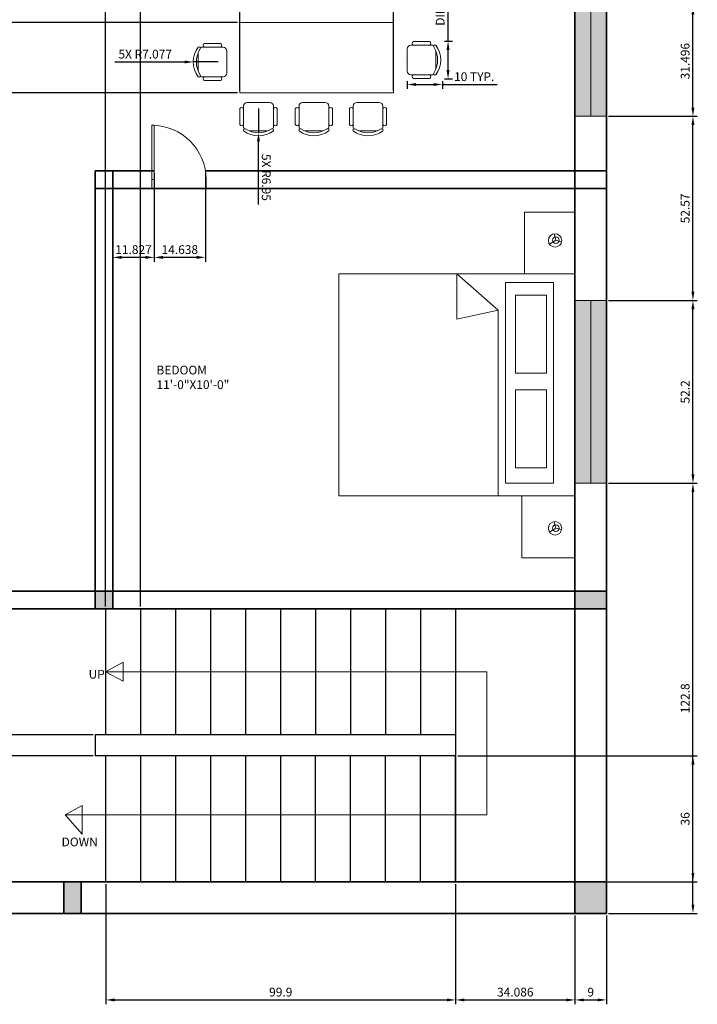
# Model space of a CAD drawing. Units: inches. Extents: x 33934 to 34340, y 20959 to 21493.
# Tile 2 of 4: x 34146 to 34340, y 20959 to 21240. Entities that reach past the tile are written whole.
import ezdxf

# ---------------------------------------------------------------- set-up
doc = ezdxf.new("R2010")
doc.units = ezdxf.units.IN
for name, color, linetype, lineweight in [('A-ANNO-DIMS', 2, 'Continuous', 18), ('A-ANNO-SYMB', 7, 'Continuous', 18), ('A-ANNO-TEXT', 7, 'Continuous', 18), ('A-AREA-IDEN', 7, 'Continuous', 18), ('A-COLS', 7, 'Continuous', 35), ('A-DOOR', 3, 'Continuous', 18), ('A-FLOR-STRS', 7, 'Continuous', 25), ('A-FURN', 8, 'Continuous', 18), ('A-GLAZ', 4, 'Continuous', 18), ('A-WALL', 7, 'Continuous', 35)]:
    doc.layers.add(name, color=color, linetype=linetype, lineweight=lineweight)
doc.layers.add('A-COLS-PATT', color=141, linetype='Continuous', lineweight=13, true_color=0xadddf7)
doc.layers.add('A-GLAZ-PATT', color=159, linetype='Continuous', lineweight=13, true_color=0x22346e)
doc.styles.get("Standard").update_dxf_attribs({"font": 'arial.ttf'})
doc.dimstyles.new('ISO-25', dxfattribs={"dimtxt": 2.5, "dimasz": 2.5, "dimexe": 1.25, "dimexo": 0.625, "dimtad": 1, "dimtxsty": 'Standard', "dimcen": 2.5, "dimadec": 0, "dimazin": 0, "dimtfac": 1, "dimtmove": 0, "dimatfit": 3, "dimfxl": 1, "dimarcsym": 0})

# ---------------------------------------------------------------- blocks, each defined once
blk = doc.blocks.new('CHAIR7')
for p, q in [((0, 9), (0, -9)), ((20, 12), (3, 12)), ((5.12, 15.04), (17.88, 15.04)), ((23, -7.44), (23, 7.44)), ((3, -12), (20, -12)), ((5.12, -15), (17.88, -15))]:
    blk.add_line(p, q)
for centre, radius, start, end in [((3, 9), 3, 90, 180), ((5.56, 13.54), 1.56, 73.7398, 286.2602), ((17.44, 13.54), 1.56, 253.7398, 106.2602), ((20, 9), 3, 62.41556, 90), ((22.34, 11.12), 1.1, 53.30994, 212.02741), ((4.82, 0), 19.64, 327.57575, 32.42425), ((7, 0), 20, 323.1301, 36.8699), ((3, -9), 3, 180, 270), ((5.56, -13.5), 1.56, 73.7398, 286.2602), ((17.44, -13.5), 1.56, 253.7398, 106.2602), ((20, -9), 3, 270, 297.58444), ((22.34, -11.12), 1.1, 147.97259, 306.69006)]:
    blk.add_arc(centre, radius, start, end)
blk = doc.blocks.new('*U5')
for p, q in [((0, 0), (0, -6)), ((40, 0), (40, -6))]:
    blk.add_line(p, q)
blk.add_lwpolyline([(0, 0), (0, 40), (1.75, 40), (1.75, 0)], close=True)
blk.add_arc((0, 0), 40, 0, 90)
blk = doc.blocks.new('BED-DOUBLE-WITH-NIGHTSTANDS')
for p, q in [((-9.63, -5.48), (-11.46, -5.95)), ((-9.63, -5.48), (-9.19, -3.82)), ((-9.63, -5.48), (-8.53, -7.28)), ((72.57, -5.48), (70.73, -5.95)), ((72.57, -5.48), (73, -3.82)), ((72.57, -5.48), (73.67, -7.28)), ((10.3, -21.96), (0, -33.74)), ((63.37, -21.96), (10.3, -21.96)), ((12.88, -33.74), (10.3, -21.96)), ((0, -33.74), (12.88, -33.74))]:
    blk.add_line(p, q)
for points in [[(-17.69, 0.01), (-0.01, 0.01), (-0.01, -14.39), (-17.69, -14.39)], [(0, 0), (63.37, 0), (63.37, -67.48), (0, -67.48)], [(63.36, 0.01), (81.04, 0.01), (81.04, -15.15), (63.36, -15.15)], [(2.46, -6.09), (59.71, -6.09), (59.71, -19.82), (2.46, -19.82)], [(6.09, -8.09), (28.36, -8.09), (28.36, -16.99), (6.09, -16.99)], [(33.05, -8.09), (55.31, -8.09), (55.31, -16.99), (33.05, -16.99)]]:
    blk.add_lwpolyline(points, close=True)
for centre, radius in [((-9.57, -5.69), 1.91), ((-9.63, -5.48), 0.951), ((72.62, -5.69), 1.91), ((72.57, -5.48), 0.951)]:
    blk.add_circle(centre, radius)
blk = doc.blocks.new('*D11')
at = {"layer": 'A-ANNO-DIMS', "color": 0, "lineweight": -2, "transparency": 16777216}
for p, q in [((34268.45, 21234.15), (34268.45, 21274.98)), ((34267.46, 21234.15), (34269.7, 21234.15)), ((34268.45, 21225.89), (34268.45, 21231.65)), ((34267.46, 21223.39), (34269.7, 21223.39))]:
    blk.add_line(p, q, dxfattribs=at)
at = {"layer": 'A-ANNO-DIMS', "color": 0, "transparency": 16777216}
for points in [[(34268.03, 21231.65), (34268.87, 21231.65), (34268.45, 21234.15)], [(34268.03, 21225.89), (34268.87, 21225.89), (34268.45, 21223.39)]]:
    blk.add_solid(points, dxfattribs=at)
at = {"layer": 'Defpoints', "color": 0, "transparency": 16777216}
for p in [(34266.83, 21234.15), (34268.45, 21234.15), (34266.83, 21223.39)]:
    blk.add_point(p, dxfattribs=at)
at = {"layer": 'A-ANNO-DIMS', "color": 0, "transparency": 16777216, "insert": (34266.53, 21255.82), "char_height": 2.5, "attachment_point": 5, "rotation": 90}
blk.add_mtext('DINING CHAIR 11 TYP.', dxfattribs=at)
blk = doc.blocks.new('*D12')
at = {"layer": 'A-ANNO-DIMS', "color": 0, "lineweight": -2, "transparency": 16777216}
for p, q in [((34256.81, 21222.77), (34256.81, 21220.53)), ((34266.83, 21222.77), (34266.83, 21220.53)), ((34259.31, 21221.78), (34264.33, 21221.78)), ((34266.83, 21221.78), (34282.52, 21221.78))]:
    blk.add_line(p, q, dxfattribs=at)
at = {"layer": 'A-ANNO-DIMS', "color": 0, "transparency": 16777216}
for points in [[(34259.31, 21222.19), (34259.31, 21221.36), (34256.81, 21221.78)], [(34264.33, 21222.19), (34264.33, 21221.36), (34266.83, 21221.78)]]:
    blk.add_solid(points, dxfattribs=at)
at = {"layer": 'Defpoints', "color": 0, "transparency": 16777216}
for p in [(34256.81, 21223.39), (34266.83, 21223.39), (34266.83, 21221.78)]:
    blk.add_point(p, dxfattribs=at)
at = {"layer": 'A-ANNO-DIMS', "color": 0, "transparency": 16777216, "insert": (34275.93, 21223.68), "char_height": 2.5, "attachment_point": 5}
blk.add_mtext('10 TYP.', dxfattribs=at)
blk = doc.blocks.new('*D23')
at = {"layer": 'A-ANNO-DIMS', "color": 0, "lineweight": -2, "transparency": 16777216}
for p, q in [((34314.32, 21107.92), (34339.64, 21107.92)), ((34338.39, 20987.61), (34338.39, 21105.42)), ((34314.32, 20985.11), (34339.64, 20985.11))]:
    blk.add_line(p, q, dxfattribs=at)
at = {"layer": 'A-ANNO-DIMS', "color": 0, "transparency": 16777216}
for points in [[(34337.98, 21105.42), (34338.81, 21105.42), (34338.39, 21107.92)], [(34337.98, 20987.61), (34338.81, 20987.61), (34338.39, 20985.11)]]:
    blk.add_solid(points, dxfattribs=at)
at = {"layer": 'Defpoints', "color": 0, "transparency": 16777216}
for p in [(34313.69, 21107.92), (34338.39, 21107.92), (34313.69, 20985.11)]:
    blk.add_point(p, dxfattribs=at)
at = {"layer": 'A-ANNO-DIMS', "color": 0, "transparency": 16777216, "insert": (34336.49, 21046.51), "char_height": 2.5, "attachment_point": 5, "rotation": 90}
blk.add_mtext('122.8', dxfattribs=at)
blk = doc.blocks.new('*D24')
at = {"layer": 'A-ANNO-DIMS', "color": 0, "lineweight": -2, "transparency": 16777216}
for p, q in [((34314.32, 21160.11), (34339.64, 21160.11)), ((34338.39, 21110.42), (34338.39, 21157.61)), ((34314.32, 21107.92), (34339.64, 21107.92))]:
    blk.add_line(p, q, dxfattribs=at)
at = {"layer": 'A-ANNO-DIMS', "color": 0, "transparency": 16777216}
for points in [[(34337.98, 21157.61), (34338.81, 21157.61), (34338.39, 21160.11)], [(34337.98, 21110.42), (34338.81, 21110.42), (34338.39, 21107.92)]]:
    blk.add_solid(points, dxfattribs=at)
at = {"layer": 'Defpoints', "color": 0, "transparency": 16777216}
for p in [(34313.69, 21160.11), (34338.39, 21160.11), (34313.69, 21107.92)]:
    blk.add_point(p, dxfattribs=at)
at = {"layer": 'A-ANNO-DIMS', "color": 0, "transparency": 16777216, "insert": (34336.49, 21134.02), "char_height": 2.5, "attachment_point": 5, "rotation": 90}
blk.add_mtext('52.2', dxfattribs=at)
blk = doc.blocks.new('*D25')
at = {"layer": 'A-ANNO-DIMS', "color": 0, "lineweight": -2, "transparency": 16777216}
for p, q in [((34314.32, 21212.69), (34339.64, 21212.69)), ((34338.39, 21162.61), (34338.39, 21210.19)), ((34314.32, 21160.11), (34339.64, 21160.11))]:
    blk.add_line(p, q, dxfattribs=at)
at = {"layer": 'A-ANNO-DIMS', "color": 0, "transparency": 16777216}
for points in [[(34337.98, 21210.19), (34338.81, 21210.19), (34338.39, 21212.69)], [(34337.98, 21162.61), (34338.81, 21162.61), (34338.39, 21160.11)]]:
    blk.add_solid(points, dxfattribs=at)
at = {"layer": 'Defpoints', "color": 0, "transparency": 16777216}
for p in [(34313.69, 21212.69), (34338.39, 21212.69), (34313.69, 21160.11)]:
    blk.add_point(p, dxfattribs=at)
at = {"layer": 'A-ANNO-DIMS', "color": 0, "transparency": 16777216, "insert": (34336.49, 21186.4), "char_height": 2.5, "attachment_point": 5, "rotation": 90}
blk.add_mtext('52.57', dxfattribs=at)
blk = doc.blocks.new('*D26')
at = {"layer": 'A-ANNO-DIMS', "color": 0, "lineweight": -2, "transparency": 16777216}
for p, q in [((34314.32, 21244.18), (34339.64, 21244.18)), ((34338.39, 21215.19), (34338.39, 21241.68)), ((34314.32, 21212.69), (34339.64, 21212.69))]:
    blk.add_line(p, q, dxfattribs=at)
at = {"layer": 'A-ANNO-DIMS', "color": 0, "transparency": 16777216}
for points in [[(34337.98, 21241.68), (34338.81, 21241.68), (34338.39, 21244.18)], [(34337.98, 21215.19), (34338.81, 21215.19), (34338.39, 21212.69)]]:
    blk.add_solid(points, dxfattribs=at)
at = {"layer": 'Defpoints', "color": 0, "transparency": 16777216}
for p in [(34313.69, 21244.18), (34338.39, 21244.18), (34313.69, 21212.69)]:
    blk.add_point(p, dxfattribs=at)
at = {"layer": 'A-ANNO-DIMS', "color": 0, "transparency": 16777216, "insert": (34336.49, 21228.44), "char_height": 2.5, "attachment_point": 5, "rotation": 90}
blk.add_mtext('31.496', dxfattribs=at)
blk = doc.blocks.new('*D29')
at = {"layer": 'A-ANNO-DIMS', "color": 0, "lineweight": -2, "transparency": 16777216}
for p, q in [((34170.7, 20993.49), (34170.7, 20959.15)), ((34270.61, 20993.49), (34270.61, 20959.15)), ((34173.2, 20960.4), (34268.11, 20960.4))]:
    blk.add_line(p, q, dxfattribs=at)
at = {"layer": 'A-ANNO-DIMS', "color": 0, "transparency": 16777216}
for points in [[(34173.2, 20960.81), (34173.2, 20959.98), (34170.7, 20960.4)], [(34268.11, 20960.81), (34268.11, 20959.98), (34270.61, 20960.4)]]:
    blk.add_solid(points, dxfattribs=at)
at = {"layer": 'Defpoints', "color": 0, "transparency": 16777216}
for p in [(34170.7, 20994.11), (34270.61, 20994.11), (34270.61, 20960.4)]:
    blk.add_point(p, dxfattribs=at)
at = {"layer": 'A-ANNO-DIMS', "color": 0, "transparency": 16777216, "insert": (34220.65, 20962.3), "char_height": 2.5, "attachment_point": 5}
blk.add_mtext('99.9', dxfattribs=at)
blk = doc.blocks.new('*D30')
at = {"layer": 'A-ANNO-DIMS', "color": 0, "lineweight": -2, "transparency": 16777216}
for p, q in [((34270.61, 20993.49), (34270.61, 20959.15)), ((34304.69, 20984.49), (34304.69, 20959.15)), ((34273.11, 20960.4), (34302.19, 20960.4))]:
    blk.add_line(p, q, dxfattribs=at)
at = {"layer": 'A-ANNO-DIMS', "color": 0, "transparency": 16777216}
for points in [[(34273.11, 20960.81), (34273.11, 20959.98), (34270.61, 20960.4)], [(34302.19, 20960.81), (34302.19, 20959.98), (34304.69, 20960.4)]]:
    blk.add_solid(points, dxfattribs=at)
at = {"layer": 'Defpoints', "color": 0, "transparency": 16777216}
for p in [(34270.61, 20994.11), (34304.69, 20985.11), (34304.69, 20960.4)]:
    blk.add_point(p, dxfattribs=at)
at = {"layer": 'A-ANNO-DIMS', "color": 0, "transparency": 16777216, "insert": (34287.65, 20962.3), "char_height": 2.5, "attachment_point": 5}
blk.add_mtext('34.086', dxfattribs=at)
blk = doc.blocks.new('*D31')
at = {"layer": 'A-ANNO-DIMS', "color": 0, "lineweight": -2, "transparency": 16777216}
for p, q in [((34271.23, 21030.11), (34339.64, 21030.11)), ((34338.39, 20996.61), (34338.39, 21027.61)), ((34271.23, 20994.11), (34339.64, 20994.11))]:
    blk.add_line(p, q, dxfattribs=at)
at = {"layer": 'A-ANNO-DIMS', "color": 0, "transparency": 16777216}
for points in [[(34337.98, 21027.61), (34338.81, 21027.61), (34338.39, 21030.11)], [(34337.98, 20996.61), (34338.81, 20996.61), (34338.39, 20994.11)]]:
    blk.add_solid(points, dxfattribs=at)
at = {"layer": 'Defpoints', "color": 0, "transparency": 16777216}
for p in [(34270.61, 21030.11), (34338.39, 21030.11), (34270.61, 20994.11)]:
    blk.add_point(p, dxfattribs=at)
at = {"layer": 'A-ANNO-DIMS', "color": 0, "transparency": 16777216, "insert": (34336.49, 21012.11), "char_height": 2.5, "attachment_point": 5, "rotation": 90}
blk.add_mtext('36', dxfattribs=at)
blk = doc.blocks.new('*D32')
at = {"layer": 'A-ANNO-DIMS', "color": 0, "lineweight": -2, "transparency": 16777216}
for p, q in [((33937.99, 21038.61), (33937.99, 21041.11)), ((34167.07, 21036.11), (33936.74, 21036.11)), ((33937.99, 21030.11), (33937.99, 21036.11)), ((34167.07, 21030.11), (33936.74, 21030.11)), ((33937.99, 21027.61), (33937.99, 21025.11))]:
    blk.add_line(p, q, dxfattribs=at)
at = {"layer": 'A-ANNO-DIMS', "color": 0, "transparency": 16777216}
for points in [[(33937.58, 21038.61), (33938.41, 21038.61), (33937.99, 21036.11)], [(33937.58, 21027.61), (33938.41, 21027.61), (33937.99, 21030.11)]]:
    blk.add_solid(points, dxfattribs=at)
at = {"layer": 'Defpoints', "color": 0, "transparency": 16777216}
for p in [(33937.99, 21036.11), (34167.69, 21036.11), (34167.69, 21030.11)]:
    blk.add_point(p, dxfattribs=at)
at = {"layer": 'A-ANNO-DIMS', "color": 0, "transparency": 16777216, "insert": (33936.09, 21033.11), "char_height": 2.5, "attachment_point": 5, "rotation": 90}
blk.add_mtext('6', dxfattribs=at)
blk = doc.blocks.new('*D33')
at = {"layer": 'A-ANNO-DIMS', "color": 0, "lineweight": -2, "transparency": 16777216}
for p, q in [((34170.61, 21072.74), (34170.61, 21491.06)), ((34173.11, 21489.81), (34178.11, 21489.81)), ((34180.61, 21072.74), (34180.61, 21491.06))]:
    blk.add_line(p, q, dxfattribs=at)
at = {"layer": 'A-ANNO-DIMS', "color": 0, "transparency": 16777216}
for points in [[(34173.11, 21490.23), (34173.11, 21489.39), (34170.61, 21489.81)], [(34178.11, 21490.23), (34178.11, 21489.39), (34180.61, 21489.81)]]:
    blk.add_solid(points, dxfattribs=at)
at = {"layer": 'Defpoints', "color": 0, "transparency": 16777216}
for p in [(34180.61, 21489.81), (34170.61, 21072.11), (34180.61, 21072.11)]:
    blk.add_point(p, dxfattribs=at)
at = {"layer": 'A-ANNO-DIMS', "color": 0, "transparency": 16777216, "insert": (34175.61, 21491.71), "char_height": 2.5, "attachment_point": 5}
blk.add_mtext('10', dxfattribs=at)
blk = doc.blocks.new('*D36')
at = {"layer": 'A-ANNO-DIMS', "color": 0, "lineweight": -2, "transparency": 16777216}
for p, q in [((34208.98, 21220.05), (34208.98, 21491.06)), ((34211.48, 21489.81), (34250.35, 21489.81)), ((34252.85, 21220.05), (34252.85, 21491.06))]:
    blk.add_line(p, q, dxfattribs=at)
at = {"layer": 'A-ANNO-DIMS', "color": 0, "transparency": 16777216}
for points in [[(34211.48, 21490.23), (34211.48, 21489.39), (34208.98, 21489.81)], [(34250.35, 21490.23), (34250.35, 21489.39), (34252.85, 21489.81)]]:
    blk.add_solid(points, dxfattribs=at)
at = {"layer": 'Defpoints', "color": 0, "transparency": 16777216}
for p in [(34252.85, 21489.81), (34208.98, 21219.43), (34252.85, 21219.43)]:
    blk.add_point(p, dxfattribs=at)
at = {"layer": 'A-ANNO-DIMS', "color": 0, "transparency": 16777216, "insert": (34230.91, 21491.71), "char_height": 2.5, "attachment_point": 5}
blk.add_mtext('43.87', dxfattribs=at)
blk = doc.blocks.new('*D37')
at = {"layer": 'A-ANNO-DIMS', "color": 0, "lineweight": -2, "transparency": 16777216}
for p, q in [((34208.35, 21239.44), (33936.74, 21239.44)), ((33937.99, 21221.93), (33937.99, 21236.94)), ((34208.35, 21219.43), (33936.74, 21219.43))]:
    blk.add_line(p, q, dxfattribs=at)
at = {"layer": 'A-ANNO-DIMS', "color": 0, "transparency": 16777216}
for points in [[(33937.58, 21236.94), (33938.41, 21236.94), (33937.99, 21239.44)], [(33937.58, 21221.93), (33938.41, 21221.93), (33937.99, 21219.43)]]:
    blk.add_solid(points, dxfattribs=at)
at = {"layer": 'Defpoints', "color": 0, "transparency": 16777216}
for p in [(33937.99, 21239.44), (34208.98, 21239.44), (34208.98, 21219.43)]:
    blk.add_point(p, dxfattribs=at)
at = {"layer": 'A-ANNO-DIMS', "color": 0, "transparency": 16777216, "insert": (33936.09, 21229.43), "char_height": 2.5, "attachment_point": 5, "rotation": 90}
blk.add_mtext('20.017', dxfattribs=at)
blk = doc.blocks.new('*D48')
at = {"layer": 'A-ANNO-DIMS', "color": 0, "lineweight": -2, "transparency": 16777216}
for p, q in [((34172.69, 21196.49), (34172.69, 21171.16)), ((34184.52, 21196.49), (34184.52, 21171.16)), ((34182.02, 21172.41), (34175.19, 21172.41))]:
    blk.add_line(p, q, dxfattribs=at)
at = {"layer": 'A-ANNO-DIMS', "color": 0, "transparency": 16777216}
for points in [[(34175.19, 21172.83), (34175.19, 21171.99), (34172.69, 21172.41)], [(34182.02, 21172.83), (34182.02, 21171.99), (34184.52, 21172.41)]]:
    blk.add_solid(points, dxfattribs=at)
at = {"layer": 'Defpoints', "color": 0, "transparency": 16777216}
for p in [(34172.69, 21197.11), (34184.52, 21197.11), (34172.69, 21172.41)]:
    blk.add_point(p, dxfattribs=at)
at = {"layer": 'A-ANNO-DIMS', "color": 0, "transparency": 16777216, "insert": (34178.61, 21174.31), "char_height": 2.5, "attachment_point": 5}
blk.add_mtext('11.827', dxfattribs=at)
blk = doc.blocks.new('*D49')
at = {"layer": 'A-ANNO-DIMS', "color": 0, "lineweight": -2, "transparency": 16777216}
for p, q in [((34184.52, 21196.49), (34184.52, 21171.16)), ((34199.16, 21196.49), (34199.16, 21171.16)), ((34196.66, 21172.41), (34187.02, 21172.41))]:
    blk.add_line(p, q, dxfattribs=at)
at = {"layer": 'A-ANNO-DIMS', "color": 0, "transparency": 16777216}
for points in [[(34187.02, 21172.83), (34187.02, 21171.99), (34184.52, 21172.41)], [(34196.66, 21172.83), (34196.66, 21171.99), (34199.16, 21172.41)]]:
    blk.add_solid(points, dxfattribs=at)
at = {"layer": 'Defpoints', "color": 0, "transparency": 16777216}
for p in [(34184.52, 21197.11), (34199.16, 21197.11), (34184.52, 21172.41)]:
    blk.add_point(p, dxfattribs=at)
at = {"layer": 'A-ANNO-DIMS', "color": 0, "transparency": 16777216, "insert": (34191.84, 21174.31), "char_height": 2.5, "attachment_point": 5}
blk.add_mtext('14.638', dxfattribs=at)
blk = doc.blocks.new('*D50')
at = {"layer": 'A-ANNO-DIMS', "color": 0, "lineweight": -2, "transparency": 16777216}
for p, q in [((34304.69, 20984.49), (34304.69, 20959.15)), ((34313.69, 20984.49), (34313.69, 20959.15)), ((34307.19, 20960.4), (34311.19, 20960.4))]:
    blk.add_line(p, q, dxfattribs=at)
at = {"layer": 'A-ANNO-DIMS', "color": 0, "transparency": 16777216}
for points in [[(34307.19, 20960.81), (34307.19, 20959.98), (34304.69, 20960.4)], [(34311.19, 20960.81), (34311.19, 20959.98), (34313.69, 20960.4)]]:
    blk.add_solid(points, dxfattribs=at)
at = {"layer": 'Defpoints', "color": 0, "transparency": 16777216}
for p in [(34304.69, 20985.11), (34313.69, 20985.11), (34313.69, 20960.4)]:
    blk.add_point(p, dxfattribs=at)
at = {"layer": 'A-ANNO-DIMS', "color": 0, "transparency": 16777216, "insert": (34309.19, 20962.3), "char_height": 2.5, "attachment_point": 5}
blk.add_mtext('9', dxfattribs=at)
blk = doc.blocks.new('*D54')
at = {"layer": 'A-ANNO-DIMS', "color": 0, "lineweight": -2, "transparency": 16777216}
for p, q in [((34173.23, 21228.21), (34193.18, 21228.21)), ((34202.75, 21228.21), (34195.68, 21228.21))]:
    blk.add_line(p, q, dxfattribs=at)
at = {"layer": 'A-ANNO-DIMS', "color": 0, "transparency": 16777216}
blk.add_solid([(34193.18, 21228.63), (34193.18, 21227.8), (34195.68, 21228.21)], dxfattribs=at)
at = {"layer": 'Defpoints', "color": 0, "transparency": 16777216}
for p in [(34195.68, 21228.21), (34202.75, 21228.21)]:
    blk.add_point(p, dxfattribs=at)
at = {"layer": 'A-ANNO-DIMS', "color": 0, "transparency": 16777216, "insert": (34181.95, 21230.12), "char_height": 2.5, "attachment_point": 5, "rotation": 359.996}
blk.add_mtext('5X R7.077', dxfattribs=at)
blk = doc.blocks.new('*D55')
at = {"layer": 'A-ANNO-DIMS', "color": 0, "lineweight": -2, "transparency": 16777216}
for p, q in [((34214.3, 21214.96), (34214.3, 21208.01)), ((34214.3, 21187.48), (34214.3, 21205.51))]:
    blk.add_line(p, q, dxfattribs=at)
at = {"layer": 'A-ANNO-DIMS', "color": 0, "transparency": 16777216}
blk.add_solid([(34214.72, 21205.51), (34213.89, 21205.51), (34214.3, 21208.01)], dxfattribs=at)
at = {"layer": 'Defpoints', "color": 0, "transparency": 16777216}
for p in [(34214.3, 21214.96), (34214.3, 21208.01)]:
    blk.add_point(p, dxfattribs=at)
at = {"layer": 'A-ANNO-DIMS', "color": 0, "transparency": 16777216, "insert": (34216.2, 21195.24), "char_height": 2.5, "attachment_point": 5, "rotation": 270.0025}
blk.add_mtext('5X R6.95', dxfattribs=at)

msp = doc.modelspace()

# ---------------------------------------------------------------- hatches: boundary and pattern name
at = {"layer": 'A-COLS-PATT'}
h = msp.add_hatch(color=256, dxfattribs=at)
h.dxf.hatch_style = 1
h.paths.add_polyline_path([(34022.6921, 20994.1104), (34013.6921, 20994.1104), (34013.6921, 20985.1104), (34022.6921, 20985.1104)])
h.paths.add_polyline_path([(34163.6921, 20994.1104), (34158.6922, 20994.1104), (34158.6922, 20985.1104), (34163.6921, 20985.1104)])
h.paths.add_polyline_path([(34313.6921, 20994.1104), (34304.6921, 20994.1104), (34304.6921, 20985.1104), (34313.6921, 20985.1104)])
h.paths.add_polyline_path([(34313.6921, 21077.1104), (34304.6921, 21077.1104), (34304.6921, 21072.1104), (34313.6921, 21072.1104)])
h.paths.add_polyline_path([(34172.6921, 21077.1104), (34167.6921, 21077.1104), (34167.6921, 21072.1104), (34172.6921, 21072.1104)])
h.paths.add_polyline_path([(34022.6921, 21324.1104), (34013.6921, 21324.1104), (34013.6921, 21318.1104), (34022.6921, 21318.1104)])
h.paths.add_polyline_path([(34171.6921, 21324.1104), (34166.6921, 21324.1104), (34166.6921, 21318.1104), (34171.6921, 21318.1104)])
h.paths.add_polyline_path([(34313.6921, 21282.1104), (34304.6921, 21282.1104), (34304.6921, 21277.1104), (34313.6921, 21277.1104)])
h.paths.add_polyline_path([(34313.6921, 21465.1104), (34304.6921, 21465.1104), (34304.6921, 21456.1104), (34313.6921, 21456.1104)])
h.paths.add_polyline_path([(34171.6921, 21465.1104), (34166.6921, 21465.1104), (34166.6921, 21456.1104), (34171.6921, 21456.1104)])
h.paths.add_polyline_path([(34022.6921, 21465.1104), (34013.6921, 21465.1104), (34013.6921, 21456.1104), (34022.6921, 21456.1104)])
at = {"layer": 'A-GLAZ-PATT'}
h = msp.add_hatch(color=256, dxfattribs=at)
h.dxf.hatch_style = 1
h.paths.add_polyline_path([(34022.6921, 21212.6089), (34018.1921, 21212.6089), (34018.1921, 21149.8921), (34022.6921, 21149.8921)])
h.paths.add_polyline_path([(34018.1921, 21212.6089), (34013.6921, 21212.6089), (34013.6921, 21149.8921), (34018.1921, 21149.8921)])
h.paths.add_polyline_path([(34142.0454, 21077.1104), (34099.5314, 21077.1104), (34099.5314, 21074.6104), (34142.0454, 21074.6104)])
h.paths.add_polyline_path([(34142.0454, 21074.6104), (34099.5314, 21074.6104), (34099.5314, 21072.1104), (34142.0454, 21072.1104)])
h.paths.add_polyline_path([(34313.6921, 21160.1148), (34309.1921, 21160.1148), (34309.1921, 21107.9155), (34313.6921, 21107.9155)])
h.paths.add_polyline_path([(34309.1921, 21160.1148), (34304.6921, 21160.1148), (34304.6921, 21107.9155), (34309.1921, 21107.9155)])
h.paths.add_polyline_path([(34309.1921, 21244.1846), (34304.6921, 21244.1846), (34304.6921, 21212.6883), (34309.1921, 21212.6883)])
h.paths.add_polyline_path([(34313.6921, 21244.1846), (34309.1921, 21244.1846), (34309.1921, 21212.6883), (34313.6921, 21212.6883)])
h.paths.add_polyline_path([(34313.6921, 21394.9809), (34309.1921, 21394.9809), (34309.1921, 21355.1902), (34313.6921, 21355.1902)])
h.paths.add_polyline_path([(34309.1921, 21394.9809), (34304.6921, 21394.9809), (34304.6921, 21355.1902), (34309.1921, 21355.1902)])
h.paths.add_polyline_path([(34257.3396, 21465.1104), (34207.5515, 21465.1104), (34207.5515, 21460.6104), (34257.3396, 21460.6104)])
h.paths.add_polyline_path([(34257.3396, 21460.6104), (34207.5515, 21460.6104), (34207.5515, 21456.1104), (34257.3396, 21456.1104)])
h.paths.add_polyline_path([(34117.2268, 21465.1104), (34063.6855, 21465.1104), (34063.6855, 21460.6104), (34117.2268, 21460.6104)])
h.paths.add_polyline_path([(34117.2268, 21460.6104), (34063.6855, 21460.6104), (34063.6855, 21456.1104), (34117.2268, 21456.1104)])
h.paths.add_polyline_path([(34022.6921, 21430.8215), (34018.1921, 21430.8215), (34018.1921, 21373.469), (34022.6921, 21373.469)])
h.paths.add_polyline_path([(34018.1921, 21430.8215), (34013.6921, 21430.8215), (34013.6921, 21373.469), (34018.1921, 21373.469)])
h.paths.add_polyline_path([(34018.1921, 21305.2021), (34013.6921, 21305.2021), (34013.6921, 21272.8905), (34018.1921, 21272.8905)])
h.paths.add_polyline_path([(34022.6921, 21305.2021), (34018.1921, 21305.2021), (34018.1921, 21272.8905), (34022.6921, 21272.8905)])

# ---------------------------------------------------------------- linework, layer by layer
at = {"layer": 'A-ANNO-SYMB'}
for p, q in [((34170.6062, 21054.1104), (34175.6822, 21056.8686)), ((34175.6822, 21056.8686), (34175.6822, 21051.3726)), ((34170.6062, 21054.1104), (34279.5369, 21054.1104)), ((34175.6822, 21051.3726), (34170.6062, 21054.1104)), ((34279.5369, 21054.1104), (34279.5369, 21013.2183)), ((34159.0541, 21013.2183), (34163.9877, 21015.9088)), ((34163.9877, 21015.9088), (34163.9877, 21007.7587)), ((34279.5369, 21013.2183), (34159.0541, 21013.2183)), ((34163.9877, 21007.7587), (34159.0541, 21013.2183))]:
    msp.add_line(p, q, dxfattribs=at)
at = {"layer": 'A-COLS'}
for p, q in [((34158.6922, 20985.0981), (34158.6922, 20994.1104)), ((34163.6921, 20994.1104), (34163.6921, 20985.1104)), ((34163.6921, 20985.1104), (34158.6922, 20985.0981))]:
    msp.add_line(p, q, dxfattribs=at)
at = {"layer": 'A-FLOR-STRS'}
for p, q in [((34170.6062, 21072.1104), (34170.6062, 21036.1104)), ((34180.6062, 21072.1104), (34180.6062, 21036.1104)), ((34190.6062, 21072.1104), (34190.6062, 21036.1104)), ((34200.6062, 21072.1104), (34200.6062, 21036.1104)), ((34210.6062, 21072.1104), (34210.6062, 21036.1104)), ((34220.6062, 21072.1104), (34220.6062, 21036.1104)), ((34230.6062, 21072.1104), (34230.6062, 21036.1104)), ((34240.6062, 21072.1104), (34240.6062, 21036.1104)), ((34250.6062, 21072.1104), (34250.6062, 21036.1104)), ((34260.6062, 21072.1104), (34260.6062, 21036.1104)), ((34270.6062, 21072.1104), (34270.6062, 20994.1104)), ((34270.6062, 21072.1104), (34270.6062, 21036.1104)), ((34270.6062, 21036.1104), (34167.6921, 21036.1104)), ((34167.6921, 21036.1104), (34167.6921, 21030.1104)), ((34270.6062, 21030.1104), (34167.6921, 21030.1104)), ((34170.6993, 20994.1104), (34170.6993, 21030.1104)), ((34180.6993, 20994.1104), (34180.6993, 21030.1104)), ((34190.6993, 20994.1104), (34190.6993, 21030.1104)), ((34200.6993, 20994.1104), (34200.6993, 21030.1104)), ((34210.6993, 20994.1104), (34210.6993, 21030.1104)), ((34220.6993, 20994.1104), (34220.6993, 21030.1104)), ((34230.6062, 20994.1104), (34230.6062, 21030.1104)), ((34240.6062, 20994.1104), (34240.6062, 21030.1104)), ((34250.6062, 20994.1104), (34250.6062, 21030.1104)), ((34260.6062, 20994.1104), (34260.6062, 21030.1104)), ((34270.6062, 20994.1104), (34270.6062, 21030.1104))]:
    msp.add_line(p, q, dxfattribs=at)
at = {"layer": 'A-FURN'}
msp.add_lwpolyline([(34208.9796, 21239.4434), (34252.8454, 21239.4434), (34252.8454, 21219.4265), (34208.9796, 21219.4265)], close=True, dxfattribs=at)
at = {"layer": 'A-GLAZ'}
for p, q in [((34309.1921, 21212.6883), (34309.1921, 21244.1846)), ((34313.6921, 21244.1846), (34313.6921, 21212.6883)), ((34313.6921, 21212.6883), (34304.6921, 21212.6883)), ((34304.6921, 21212.6883), (34309.1921, 21212.6883)), ((34304.6921, 21160.1148), (34313.6921, 21160.1148)), ((34309.1921, 21107.9155), (34309.1921, 21160.1148)), ((34313.6921, 21160.1148), (34313.6921, 21107.9155)), ((34313.6921, 21107.9155), (34304.6921, 21107.9155)), ((34304.6921, 21107.9155), (34309.1921, 21107.9155))]:
    msp.add_line(p, q, dxfattribs=at)
at = {"layer": 'A-WALL'}
for p, q in [((34313.6921, 21465.1104), (34313.6921, 20985.1104)), ((34304.6921, 21257.1104), (34304.6921, 20985.1104)), ((34167.6921, 21197.1104), (34167.6921, 21072.1104)), ((34184.519, 21197.1104), (34167.6921, 21197.1104)), ((34172.6921, 21197.1104), (34172.6921, 21072.1104)), ((34313.6921, 21197.1104), (34199.1566, 21197.1104)), ((34313.6921, 21192.1104), (34167.6921, 21192.1104)), ((34167.6921, 21077.1104), (34075.2088, 21077.1104)), ((34313.6921, 21077.1104), (34167.6921, 21077.1104)), ((34313.6921, 21072.1104), (34075.2088, 21072.1104)), ((34313.6921, 20994.1104), (34013.6921, 20994.1104)), ((34313.6921, 20985.1104), (34013.6921, 20985.1104))]:
    msp.add_line(p, q, dxfattribs=at)

# ---------------------------------------------------------------- block references
at = {"layer": 'A-DOOR', "xscale": 0.3880097502641484, "yscale": 0.3880097502641484, "zscale": 0.3880097502641484}
msp.add_blockref('*U5', (34183.84, 21194.6032), dxfattribs=at)
at = {"layer": 'A-FURN', "xscale": 0.353847974837975, "yscale": 0.353847974837975, "zscale": 0.353847974837975}
msp.add_blockref('CHAIR7', (34256.8085, 21228.7643), dxfattribs=at)
for p, rotation in [((34205.2305, 21228.2125), 180), ((34214.3027, 21216.6635), 270), ((34230.1325, 21216.6635), 270), ((34245.5813, 21216.6635), 270)]:
    msp.add_blockref('CHAIR7', p, dxfattribs=dict(at, rotation=rotation))
at = {"layer": 'A-FURN', "rotation": 270.0000000000437}
msp.add_blockref('BED-DOUBLE-WITH-NIGHTSTANDS', (34304.6921, 21167.6717), dxfattribs=at)

# ---------------------------------------------------------------- texts
at = {"layer": 'A-ANNO-TEXT', "char_height": 2.5, "attachment_point": 1}
for s, width, insert in [('UP', 3.59236, (34165.7719, 21054.637)), ('DOWN', 10.685362, (34158.0761, 21006.752))]:
    msp.add_mtext_dynamic_manual_height_columns(s, width=width, gutter_width=12.5, heights=[0], dxfattribs=dict(at, insert=insert))
at = {"layer": 'A-AREA-IDEN', "insert": (34185.1679, 21141.489), "char_height": 2.5, "attachment_point": 1}
msp.add_mtext_dynamic_manual_height_columns('BEDOOM\\P11\'-0"X10\'-0"', width=41.705732, gutter_width=12.5, heights=[0], dxfattribs=at)

# ---------------------------------------------------------------- dimensions: what is measured, and where the dimension line sits
at = {"layer": 'A-ANNO-DIMS'}
for base, p1, p2, override, picture, middle in [((34180.6062, 21489.8104), (34170.6062, 21072.1104), (34180.6062, 21072.1104), {"dimdec": 0, "dimlfac": 1, "dimrnd": 0, "dimzin": 0, "dimdsep": 46, "dimlunit": 2}, '*D33', (34175.6062, 21491.7119)), ((34252.8454, 21489.8104), (34208.9796, 21219.4265), (34252.8454, 21219.4265), {"dimdec": 2, "dimlfac": 1, "dimrnd": 0, "dimzin": 0, "dimdsep": 46, "dimlunit": 2}, '*D36', (34230.9125, 21491.7127)), ((34270.6062, 20960.3981), (34170.6993, 20994.1104), (34270.6062, 20994.1104), {"dimdec": 1, "dimlfac": 1, "dimrnd": 0, "dimzin": 0, "dimdsep": 46, "dimlunit": 2}, '*D29', (34220.6527, 20962.2995)), ((34304.6921, 20960.3981), (34270.6062, 20994.1104), (34304.6921, 20985.1104), {"dimdec": 3, "dimlfac": 1, "dimrnd": 0, "dimzin": 0, "dimdsep": 46, "dimlunit": 2}, '*D30', (34287.6492, 20962.3004)), ((34313.6921, 20960.3981), (34304.6921, 20985.1104), (34313.6921, 20985.1104), {"dimdec": 0, "dimlfac": 1, "dimrnd": 0, "dimzin": 0, "dimdsep": 46, "dimlunit": 2}, '*D50', (34309.1921, 20962.2995))]:
    dim = msp.add_linear_dim(base=base, p1=p1, p2=p2, dimstyle='ISO-25', override=override, dxfattribs=at)
    dim.commit()
    dim.dimension.update_dxf_attribs({"geometry": picture, "text_midpoint": middle})
dim = msp.add_linear_dim(base=(34268.4486, 21234.1528), p1=(34266.8342, 21223.3907), p2=(34266.8342, 21234.1528), angle=90, text='DINING CHAIR <> TYP.', dimstyle='ISO-25', override={"dimdec": 0, "dimlfac": 1, "dimrnd": 0, "dimzin": 0, "dimdsep": 46, "dimlunit": 2}, dxfattribs=at)
dim.commit()
dim.dimension.update_dxf_attribs({"geometry": '*D11', "text_midpoint": (34266.5309, 21255.8155)})
for base, p1, p2, angle, override, picture, middle in [((34338.3921, 21244.1846), (34313.6921, 21212.6883), (34313.6921, 21244.1846), 90, {"dimdec": 3, "dimlfac": 1, "dimrnd": 0, "dimzin": 0, "dimdsep": 46, "dimlunit": 2}, '*D26', (34336.4899, 21228.4364)), ((33937.9921, 21239.4434), (34208.9796, 21219.4265), (34208.9796, 21239.4434), 90, {"dimdec": 3, "dimlfac": 1, "dimrnd": 0, "dimzin": 0, "dimdsep": 46, "dimlunit": 2}, '*D37', (33936.0907, 21229.4349)), ((34338.3921, 21212.6883), (34313.6921, 21160.1148), (34313.6921, 21212.6883), 90, {"dimdec": 2, "dimlfac": 1, "dimrnd": 0, "dimzin": 0, "dimdsep": 46, "dimlunit": 2}, '*D25', (34336.4907, 21186.4015)), ((34172.6921, 21172.4104), (34184.519, 21197.1104), (34172.6921, 21197.1104), 180, {"dimdec": 3, "dimlfac": 1, "dimrnd": 0, "dimzin": 0, "dimdsep": 46, "dimlunit": 2}, '*D48', (34178.6056, 21174.3119)), ((34184.519, 21172.4104), (34199.1566, 21197.1104), (34184.519, 21197.1104), 180, {"dimdec": 3, "dimlfac": 1, "dimrnd": 0, "dimzin": 0, "dimdsep": 46, "dimlunit": 2}, '*D49', (34191.8378, 21174.3127)), ((34338.3921, 21160.1148), (34313.6921, 21107.9155), (34313.6921, 21160.1148), 90, {"dimdec": 1, "dimlfac": 1, "dimrnd": 0, "dimzin": 0, "dimdsep": 46, "dimlunit": 2}, '*D24', (34336.4907, 21134.0151)), ((34338.3921, 21107.9155), (34313.6921, 20985.1104), (34313.6921, 21107.9155), 90, {"dimdec": 1, "dimlfac": 1, "dimrnd": 0, "dimzin": 0, "dimdsep": 46, "dimlunit": 2}, '*D23', (34336.4907, 21046.513)), ((33937.9921, 21036.1104), (34167.6921, 21030.1104), (34167.6921, 21036.1104), 90, {"dimdec": 0, "dimlfac": 1, "dimrnd": 0, "dimzin": 0, "dimdsep": 46, "dimlunit": 2}, '*D32', (33936.0907, 21033.1104)), ((34338.3921, 21030.1104), (34270.6062, 20994.1104), (34270.6062, 21030.1104), 90, {"dimdec": 0, "dimlfac": 1, "dimrnd": 0, "dimzin": 0, "dimdsep": 46, "dimlunit": 2}, '*D31', (34336.4899, 21012.1104))]:
    dim = msp.add_linear_dim(base=base, p1=p1, p2=p2, angle=angle, dimstyle='ISO-25', override=override, dxfattribs=at)
    dim.commit()
    dim.dimension.update_dxf_attribs({"geometry": picture, "text_midpoint": middle})
for center, mpoint, override, picture, middle in [((34202.7536, 21228.2125), (34195.6766, 21228.213), {"dimdec": 3, "dimlfac": 1, "dimrnd": 0, "dimzin": 0, "dimdsep": 46, "dimlunit": 2}, '*D54', (34181.9515, 21230.1154)), ((34214.3027, 21214.9567), (34214.303, 21208.0071), {"dimdec": 2, "dimlfac": 1, "dimrnd": 0, "dimzin": 0, "dimdsep": 46, "dimlunit": 2}, '*D55', (34216.205, 21195.2437))]:
    dim = msp.add_radius_dim(center=center, mpoint=mpoint, text='5X <>', dimstyle='ISO-25', override=override, dxfattribs=at)
    dim.commit()
    dim.dimension.update_dxf_attribs({"geometry": picture, "text_midpoint": middle})
dim = msp.add_linear_dim(base=(34266.8342, 21221.7764), p1=(34256.8085, 21223.3907), p2=(34266.8342, 21223.3907), text='<> TYP.', dimstyle='ISO-25', override={"dimdec": 0, "dimlfac": 1, "dimrnd": 0, "dimzin": 0, "dimdsep": 46, "dimlunit": 2}, dxfattribs=at)
dim.commit()
dim.dimension.update_dxf_attribs({"geometry": '*D12', "text_midpoint": (34275.9262, 21223.6778)})

doc.saveas('drawing.dxf')
